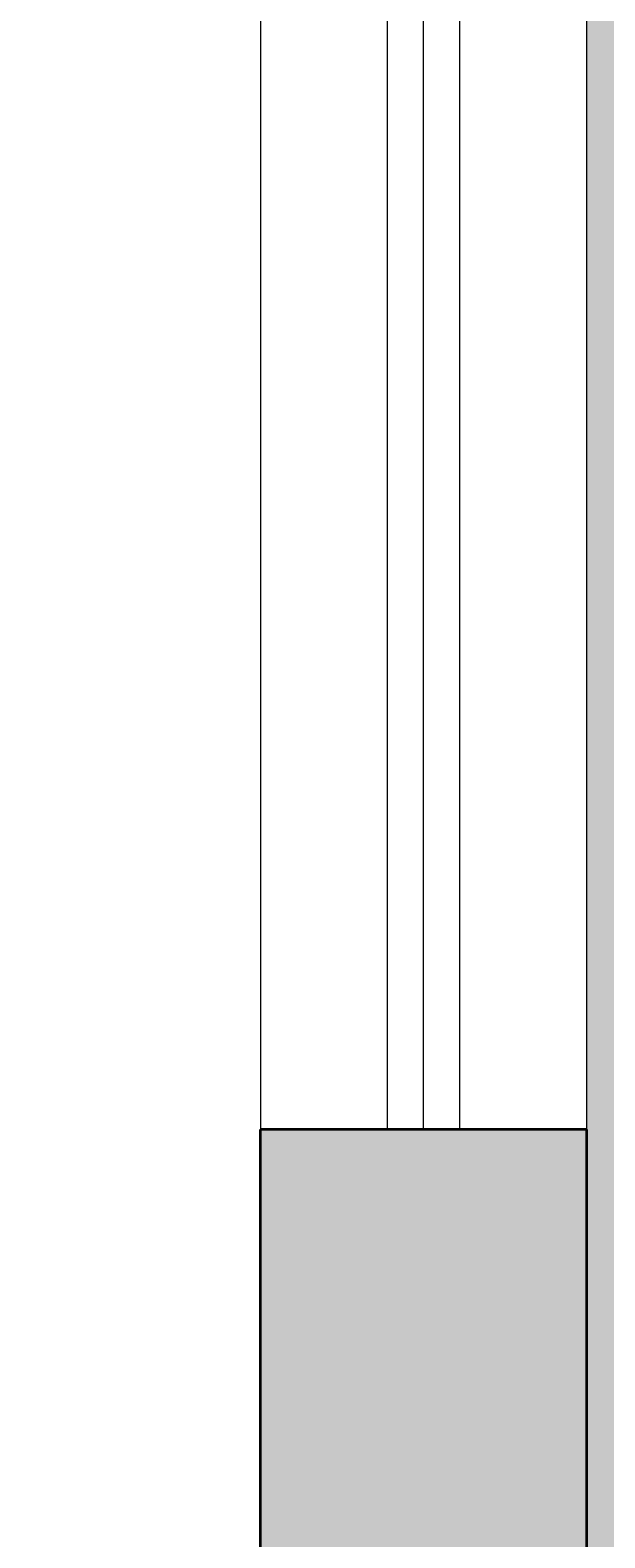
# Model space of a CAD drawing. Units: inches. Extents: x 84 to 1044, y -280 to 906.
# Tile 69 of 105: x 689 to 705, y 408 to 450. Entities that reach past the tile are written whole.
import ezdxf

# ---------------------------------------------------------------- set-up
doc = ezdxf.new("R2010")
doc.units = ezdxf.units.IN
for name, color, linetype, lineweight in [('A-ANNO-DIMS', 2, 'Continuous', 18), ('WALL', 250, 'Continuous', 35), ('WINDOW', 160, 'Continuous', 13)]:
    doc.layers.add(name, color=color, linetype=linetype, lineweight=lineweight)
doc.layers.add('A-WALL-PATT', color=251, linetype='Continuous', lineweight=9, true_color=0x636466)
doc.layers.add('L-PLNT-PATT', color=9, linetype='Continuous', lineweight=9, true_color=0xafd9aa)
doc.styles.get("Standard").update_dxf_attribs({"font": 'arial.ttf'})
doc.dimstyles.get("Standard").update_dxf_attribs({"dimtxt": 0.18, "dimasz": 0.18, "dimexe": 0.18, "dimexo": 0.0625, "dimgap": 0.09, "dimtad": 0, "dimtih": 1, "dimtoh": 1, "dimdec": 4, "dimzin": 0, "dimdsep": 46, "dimtxsty": 'Standard', "dimcen": 0.09, "dimadec": 0, "dimazin": 0, "dimtfac": 1, "dimtdec": 4, "dimtofl": 0, "dimtmove": 0, "dimatfit": 3, "dimfxl": 1, "dimtolj": 1, "dimtzin": 0, "dimarcsym": 0})

# ---------------------------------------------------------------- blocks, each defined once
blk = doc.blocks.new('WIN-72IN')
for p, q in [((72.004, 9), (0.004, 9)), ((72.004, 5.5), (0.004, 5.5)), ((72.004, 4.5), (0.004, 4.5)), ((72.004, 3.5), (0.004, 3.5)), ((0.004, 0), (72.004, 0))]:
    blk.add_line(p, q)
blk = doc.blocks.new('*D62')
at = {"layer": 'A-ANNO-DIMS', "color": 0, "lineweight": -2, "transparency": 16777216}
for p, q in [((203.179, 709.183), (203.179, 905.9)), ((203.359, 905.72), (549.232, 905.72)), ((895.894, 905.72), (550.021, 905.72)), ((896.074, 400.183), (896.074, 905.9))]:
    blk.add_line(p, q, dxfattribs=at)
at = {"layer": 'A-ANNO-DIMS', "color": 0, "transparency": 16777216}
for points in [[(203.359, 905.75), (203.359, 905.69), (203.179, 905.72)], [(895.894, 905.75), (895.894, 905.69), (896.074, 905.72)]]:
    blk.add_solid(points, dxfattribs=at)
at = {"layer": 'Defpoints', "color": 0, "transparency": 16777216}
for p in [(896.074, 905.72), (203.179, 709.12), (896.074, 400.12)]:
    blk.add_point(p, dxfattribs=at)
at = {"layer": 'A-ANNO-DIMS', "color": 0, "transparency": 16777216, "insert": (549.627, 905.72), "char_height": 0.18, "attachment_point": 5}
blk.add_mtext('\\A1;692.9', dxfattribs=at)

msp = doc.modelspace()

# ---------------------------------------------------------------- hatches: boundary and pattern name
at = {"layer": 'A-WALL-PATT', "transparency": 33554597}
h = msp.add_hatch(color=256, dxfattribs=at)
h.dxf.hatch_style = 1
h.paths.add_polyline_path([(671.074, 100.12), (647.074, 100.12), (647.074, 160.12), (641.074, 160.12), (620.824, 160.12), (620.824, 151.12), (638.074, 151.12), (638.074, 91.12), (671.074, 91.12)])
h.paths.add_polyline_path([(791.074, 100.12), (743.074, 100.12), (743.074, 91.12), (791.074, 91.12)])
h.paths.add_polyline_path([(896.074, 346.12), (887.074, 346.12), (887.074, 334.12), (870.955, 334.12), (833.074, 334.12), (804.574, 334.12), (804.574, 328.12), (887.074, 328.12), (887.074, 100.12), (863.074, 100.12), (863.074, 91.12), (896.074, 91.12)])
h.paths.add_polyline_path([(507.574, 154.729), (507.574, 160.12), (464.074, 160.12), (464.074, 247.12), (641.074, 247.12), (641.074, 208.12), (647.074, 208.12), (647.074, 328.12), (659.074, 328.12), (659.074, 334.12), (617.074, 334.12), (617.074, 328.12), (641.074, 328.12), (641.074, 256.12), (545.074, 256.12), (545.074, 328.12), (569.074, 328.12), (569.074, 334.12), (518.074, 334.12), (518.074, 325.12), (536.074, 325.12), (536.074, 256.12), (464.074, 256.12), (464.074, 325.12), (482.074, 325.12), (482.074, 334.12), (455.074, 334.12), (455.074, 160.12), (413.127, 160.12), (413.127, 151.12), (455.074, 151.12), (455.074, 91.12), (464.074, 91.12), (464.074, 151.12), (507.574, 151.12)])
h.paths.add_polyline_path([(572.824, 160.12), (555.574, 160.12), (555.574, 151.12), (572.824, 151.12)], flags=17)
h.paths.add_polyline_path([(341.127, 160.12), (299.179, 160.12), (299.179, 211.12), (294.179, 211.12), (290.179, 211.12), (290.179, 151.12), (341.127, 151.12)])
h.paths.add_polyline_path([(299.179, 256.12), (212.179, 256.12), (212.179, 274.12), (203.179, 274.12), (203.179, 247.12), (299.179, 247.12)])
h.paths.add_polyline_path([(212.179, 514.12), (398.074, 514.12), (398.074, 519.12), (398.074, 520.12), (212.179, 520.12), (212.179, 574.12), (203.179, 574.12), (203.179, 310.12), (212.179, 310.12), (212.179, 328.12), (290.179, 328.12), (290.179, 292.12), (299.179, 292.12), (299.179, 328.12), (332.179, 328.12), (332.179, 334.12), (212.179, 334.12)])
h.paths.add_polyline_path([(287.127, 709.12), (203.179, 709.12), (203.179, 646.12), (212.179, 646.12), (212.179, 700.12), (287.127, 700.12)])
h.paths.add_polyline_path([(470.074, 709.12), (359.127, 709.12), (359.127, 700.12), (434.074, 700.12), (434.074, 574.12), (440.074, 574.12), (440.074, 622.12), (464.074, 622.12), (464.074, 628.12), (440.074, 628.12), (440.074, 700.12), (470.074, 700.12)])
h.paths.add_polyline_path([(572.074, 709.12), (506.074, 709.12), (506.074, 700.12), (536.074, 700.12), (536.074, 628.12), (494.074, 628.12), (494.074, 622.12), (536.074, 622.12), (536.074, 520.12), (440.074, 520.12), (440.074, 544.12), (434.074, 544.12), (434.074, 514.12), (644.074, 514.12), (644.074, 519.12), (644.074, 544.12), (638.074, 544.12), (638.074, 520.12), (542.074, 520.12), (542.074, 622.12), (584.074, 622.12), (584.074, 628.12), (542.074, 628.12), (542.074, 700.12), (572.074, 700.12)])
h.paths.add_polyline_path([(698.074, 709.12), (608.074, 709.12), (608.074, 700.12), (638.074, 700.12), (638.074, 628.12), (614.074, 628.12), (614.074, 622.12), (638.074, 622.12), (638.074, 574.12), (644.074, 574.12), (644.074, 700.12), (698.074, 700.12)])
h.paths.add_polyline_path([(833.074, 709.12), (770.074, 709.12), (770.074, 700.12), (824.074, 700.12), (824.074, 646.12), (833.074, 646.12)])
h.paths.add_polyline_path([(833.074, 574.12), (824.074, 574.12), (824.074, 520.12), (791.244, 520.12), (712.904, 520.12), (680.074, 520.12), (680.074, 514.12), (695.074, 514.12), (695.074, 491.62), (704.074, 491.62), (704.074, 511.12), (833.074, 511.12)])
h.paths.add_polyline_path([(704.074, 419.62), (695.074, 419.62), (695.074, 370.12), (704.074, 370.12)])
h.paths.add_polyline_path([(896.074, 400.12), (833.074, 400.12), (833.074, 364.12), (839.074, 364.12), (839.074, 394.12), (887.074, 394.12), (887.074, 382.12), (896.074, 382.12)])
h.paths.add_polyline_path([(732.574, 334.12), (695.074, 334.12), (695.074, 328.12), (732.574, 328.12)])
at = {"layer": 'L-PLNT-PATT', "transparency": 33554597}
h = msp.add_hatch(color=256, dxfattribs=at)
h.dxf.hatch_style = 1
h.paths.add_polyline_path([(896.074, 511.12), (704.074, 511.12), (704.074, 491.62), (704.074, 419.62), (704.074, 400.12), (833.074, 400.12), (896.074, 400.12)])

# ---------------------------------------------------------------- linework, layer by layer
at = {"layer": 'WALL'}
for p, q in [((704.074, 419.62), (695.074, 419.62)), ((695.074, 370.12), (695.074, 419.62)), ((704.074, 370.12), (704.074, 419.62))]:
    msp.add_line(p, q, dxfattribs=at)

# ---------------------------------------------------------------- block references
at = {"layer": 'WINDOW', "rotation": 270.0000000000001}
msp.add_blockref('WIN-72IN', (695.074, 491.624), dxfattribs=at)

# ---------------------------------------------------------------- dimensions: what is measured, and where the dimension line sits
at = {"layer": 'A-ANNO-DIMS'}
dim = msp.add_linear_dim(base=(896.074, 905.72), p1=(203.179, 709.12), p2=(896.074, 400.12), dimstyle='Standard', override={"dimdec": 1, "dimlfac": 1, "dimrnd": 0, "dimzin": 0, "dimdsep": 46, "dimlunit": 2}, dxfattribs=at)
dim.commit()
dim.dimension.update_dxf_attribs({"geometry": '*D62', "text_midpoint": (549.627, 905.72)})

doc.saveas('drawing.dxf')
